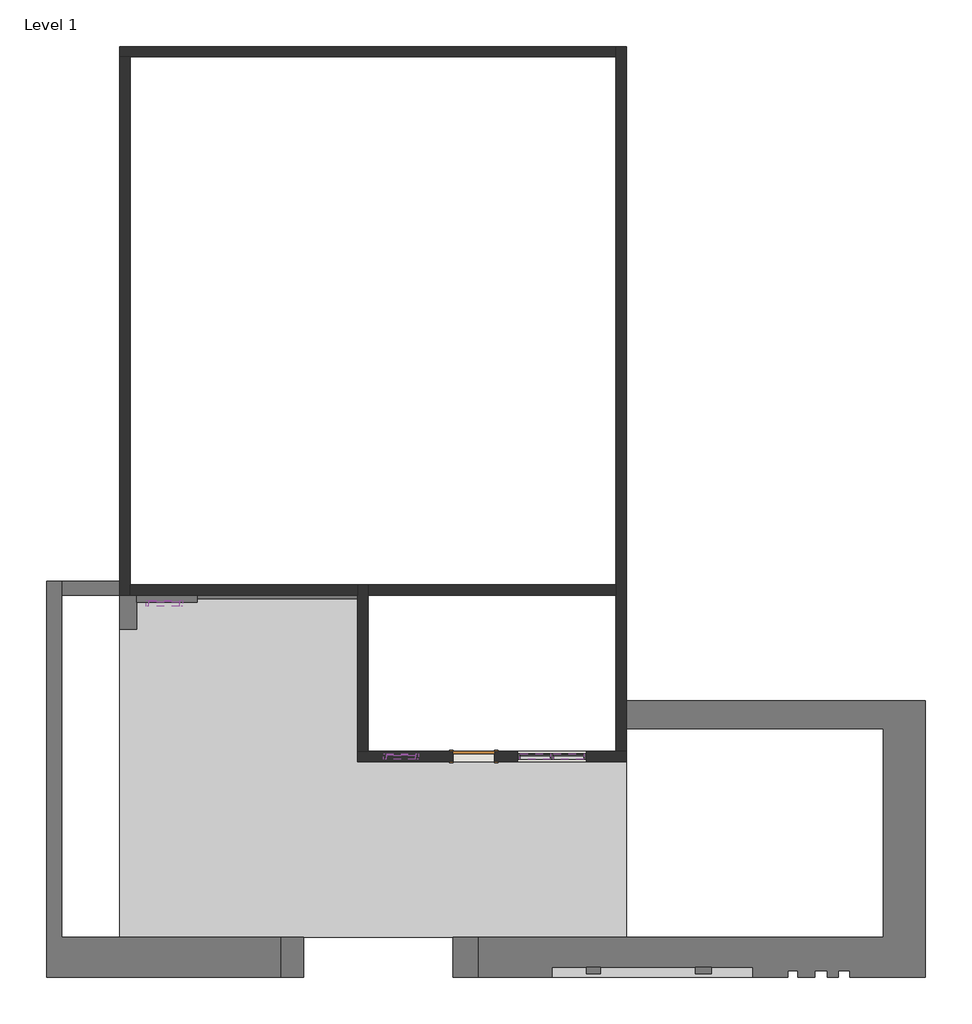
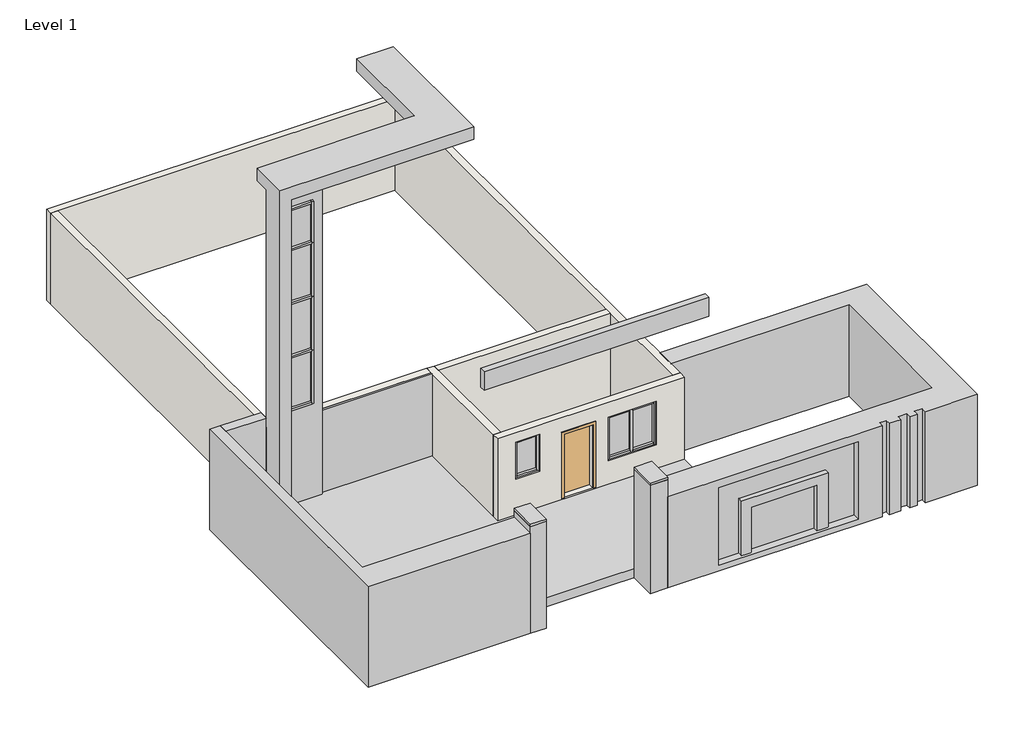
# One storey: 24 members, 7 plates, 7 walls, 4 proxies, 1 door.
"""IFC4 building model written with IfcOpenShell, lengths in millimetres."""

from ifc_helpers import new_model, si_unit, origin, origin_with_axes, place, context, project, spatial, polyline, outline, extrude, faceted_brep, transform, mapped, element, save
from components import generic_models_3_generic_models_3_20a2e421, generic_models_4_generic_models_4_e8bbcad5, generic_models_5_generic_models_5_9540ccd6, door_0ca8825f, member_c33c434a, member_9369ce3c, member_269047fe, member_5e365d0c, member_2caf7d25, member_5295ae1b, member_af550d70, member_0a83a24a, member_c6627131, system_panel_glazed_125786c9, system_panel_glazed_5a872b22, system_panel_glazed_70269732, system_panel_glazed_db295b58, system_panel_glazed_980f9714

model = new_model("IFC4")

# Units and contexts
model_context = context("Model", 3, world=origin())
ifc_project = project(units=[si_unit("LENGTHUNIT", "METRE", prefix="MILLI")], contexts=[model_context])

# Site, building, storey
site = spatial("IfcSite", under=ifc_project)
building = spatial("IfcBuilding", under=site)
storey = spatial("IfcBuildingStorey", under=building, Name="Level 1", Elevation=0.0)

# Proxies
placement = place(None, origin())
element("IfcBuildingElementProxy", 1, Name="Generic Models 1 : Generic Models 1", ObjectType="Generic Models 1 : Generic Models 1", at=placement, inside=storey, context=model_context, shape_type="Brep", body=[
    faceted_brep([(-10657.4321088, -9400.4468404, 304.8), (-15877.1321088, -9400.4468404, 304.8), (-15877.1321088, -16906.1468404, 304.8), (-4751.9321088, -16906.1468404, 304.8), (-4751.9321088, -13058.0468404, 304.8), (-10657.4321088, -13058.0468404, 304.8), (-10657.4321088, -12829.4468404, 304.8), (-10657.4321088, -13058.0468404, 0.0), (-4751.9321088, -13058.0468404, 0.0), (-4751.9321088, -16906.1468404, 0.0), (-15877.1321088, -16906.1468404, 0.0), (-15877.1321088, -9400.4468404, 0.0), (-10657.4321088, -9400.4468404, 0.0), (-10657.4321088, -12829.4468404, 0.0)], [[[0, 1, 2, 3, 4, 5, 6]], [[7, 8, 9, 10, 11, 12, 13]], [[1, 0, 12, 11]], [[2, 1, 11, 10]], [[12, 0, 6, 5, 7, 13]], [[3, 2, 10, 9]], [[4, 3, 9, 8]], [[5, 4, 8, 7]]]),
])
generic_models_3_generic_models_3_shape = generic_models_3_generic_models_3_20a2e421(model_context)
element("IfcBuildingElementProxy", 2, Name="Generic Models 3 : Generic Models 3", ObjectType="Generic Models 3 : Generic Models 3", at=placement, inside=storey, context=model_context, shape_type="MappedRepresentation", body=[
    mapped(generic_models_3_generic_models_3_shape, transform((0.0, 0.0, 0.0), x_axis=(1.0, 0.0, 0.0), y_axis=(0.0, 1.0, 0.0), z_axis=(0.0, 0.0, 1.0))),
])
generic_models_4_generic_models_4_shape = generic_models_4_generic_models_4_e8bbcad5(model_context)
element("IfcBuildingElementProxy", 3, Name="Generic Models 4 : Generic Models 4", ObjectType="Generic Models 4 : Generic Models 4", at=placement, inside=storey, context=model_context, shape_type="MappedRepresentation", body=[
    mapped(generic_models_4_generic_models_4_shape, transform((0.0, 0.0, 0.0), x_axis=(1.0, 0.0, 0.0), y_axis=(0.0, 1.0, 0.0), z_axis=(0.0, 0.0, 1.0))),
])
generic_models_5_generic_models_5_shape = generic_models_5_generic_models_5_9540ccd6(model_context)
element("IfcBuildingElementProxy", 4, Name="Generic Models 5 : Generic Models 5", ObjectType="Generic Models 5 : Generic Models 5", at=placement, inside=storey, context=model_context, shape_type="MappedRepresentation", body=[
    mapped(generic_models_5_generic_models_5_shape, transform((0.0, 0.0, 0.0), x_axis=(1.0, 0.0, 0.0), y_axis=(0.0, 1.0, 0.0), z_axis=(0.0, 0.0, 1.0))),
])

# Door
door_shape = door_0ca8825f(model_context)
element("IfcDoor", 5, ObjectType="Single-Flush : 36\" x 84\"", at=placement, inside=storey, context=model_context, shape_type="MappedRepresentation", body=[
    mapped(door_shape, transform((-8104.7321088, -12943.7468404, 355.6), x_axis=(1.0, 0.0, 0.0), y_axis=(0.0, 1.0, 0.0), z_axis=(0.0, 0.0, 1.0))),
])

# Members
member_shape = member_c33c434a(model_context)
element("IfcMember", 6, ObjectType="Rectangular Mullion : 2.5\" x 5\" rectangular", at=placement, inside=storey, context=model_context, shape_type="MappedRepresentation", body=[
    mapped(member_shape, transform((-6358.4821088, -12943.7468404, 1083.0066443), x_axis=(0.0, 0.0, -1.0), y_axis=(0.0, -1.0, 0.0), z_axis=(-1.0, 0.0, 0.0))),
])
element("IfcMember", 7, ObjectType="Rectangular Mullion : 2.5\" x 5\" rectangular", at=placement, inside=storey, context=model_context, shape_type="MappedRepresentation", body=[
    mapped(member_shape, transform((-7088.7321088, -12943.7468404, 1083.0066443), x_axis=(0.0, 0.0, -1.0), y_axis=(0.0, -1.0, 0.0), z_axis=(-1.0, 0.0, 0.0))),
])
member_2_shape = member_9369ce3c(model_context)
element("IfcMember", 8, ObjectType="Rectangular Mullion : 2.5\" x 5\" rectangular", at=placement, inside=storey, context=model_context, shape_type="MappedRepresentation", body=[
    mapped(member_2_shape, transform((-6390.2321088, -12943.7468404, 1083.0066443), x_axis=(1.0, 0.0, 0.0), y_axis=(0.0, -1.0, 0.0), z_axis=(0.0, 0.0, -1.0))),
])
element("IfcMember", 9, ObjectType="Rectangular Mullion : 2.5\" x 5\" rectangular", at=placement, inside=storey, context=model_context, shape_type="MappedRepresentation", body=[
    mapped(member_shape, transform((-6421.9821088, -12943.7468404, 2538.9721274), x_axis=(0.0, 0.0, 1.0), y_axis=(0.0, -1.0, 0.0), z_axis=(1.0, 0.0, 0.0))),
])
element("IfcMember", 10, ObjectType="Rectangular Mullion : 2.5\" x 5\" rectangular", at=placement, inside=storey, context=model_context, shape_type="MappedRepresentation", body=[
    mapped(member_shape, transform((-5691.7321088, -12943.7468404, 2538.9721274), x_axis=(0.0, 0.0, 1.0), y_axis=(0.0, -1.0, 0.0), z_axis=(1.0, 0.0, 0.0))),
])
member_3_shape = member_269047fe(model_context)
element("IfcMember", 11, ObjectType="Rectangular Mullion : 2.5\" x 5\" rectangular", at=placement, inside=storey, context=model_context, shape_type="MappedRepresentation", body=[
    mapped(member_3_shape, transform((-7152.2321088, -12943.7468404, 2538.9721274), x_axis=(-1.0, 0.0, 0.0), y_axis=(0.0, -1.0, 0.0), z_axis=(0.0, 0.0, 1.0))),
])
element("IfcMember", 12, ObjectType="Rectangular Mullion : 2.5\" x 5\" rectangular", at=placement, inside=storey, context=model_context, shape_type="MappedRepresentation", body=[
    mapped(member_3_shape, transform((-5628.2321088, -12943.7468404, 1083.0066443), x_axis=(1.0, 0.0, 0.0), y_axis=(0.0, -1.0, 0.0), z_axis=(0.0, 0.0, -1.0))),
])
member_4_shape = member_5e365d0c(model_context)
element("IfcMember", 13, ObjectType="Rectangular Mullion : 2.5\" x 5\" rectangular", at=placement, inside=storey, context=model_context, shape_type="MappedRepresentation", body=[
    mapped(member_4_shape, transform((-10022.4321088, -12943.7468404, 1497.0984453), x_axis=(0.0, 0.0, -1.0), y_axis=(0.0, -1.0, 0.0), z_axis=(-1.0, 0.0, 0.0))),
])
element("IfcMember", 14, ObjectType="Rectangular Mullion : 2.5\" x 5\" rectangular", at=placement, inside=storey, context=model_context, shape_type="MappedRepresentation", body=[
    mapped(member_4_shape, transform((-9387.4321088, -12943.7468404, 2733.8418528), x_axis=(0.0, 0.0, 1.0), y_axis=(0.0, -1.0, 0.0), z_axis=(1.0, 0.0, 0.0))),
])
member_5_shape = member_2caf7d25(model_context)
element("IfcMember", 15, ObjectType="Rectangular Mullion : 2.5\" x 5\" rectangular", at=placement, inside=storey, context=model_context, shape_type="MappedRepresentation", body=[
    mapped(member_5_shape, transform((-10085.9321088, -12943.7468404, 2733.8418528), x_axis=(-1.0, 0.0, 0.0), y_axis=(0.0, -1.0, 0.0), z_axis=(0.0, 0.0, 1.0))),
])
element("IfcMember", 16, ObjectType="Rectangular Mullion : 2.5\" x 5\" rectangular", at=placement, inside=storey, context=model_context, shape_type="MappedRepresentation", body=[
    mapped(member_5_shape, transform((-9323.9321088, -12943.7468404, 1497.0984453), x_axis=(1.0, 0.0, 0.0), y_axis=(0.0, -1.0, 0.0), z_axis=(0.0, 0.0, -1.0))),
])
member_6_shape = member_5295ae1b(model_context)
element("IfcMember", 17, ObjectType="Rectangular Mullion : 2.5\" x 5\" rectangular", at=placement, inside=storey, context=model_context, shape_type="MappedRepresentation", body=[
    mapped(member_6_shape, transform((-15305.6321088, -9579.3158046, 7104.8631502), x_axis=(-1.0, 0.0, 0.0), y_axis=(0.0, -1.0, 0.0), z_axis=(0.0, 0.0, 1.0))),
])
element("IfcMember", 18, ObjectType="Rectangular Mullion : 2.5\" x 5\" rectangular", at=placement, inside=storey, context=model_context, shape_type="MappedRepresentation", body=[
    mapped(member_6_shape, transform((-15305.6321088, -9579.3158046, 8903.6180215), x_axis=(-1.0, 0.0, 0.0), y_axis=(0.0, -1.0, 0.0), z_axis=(0.0, 0.0, 1.0))),
])
member_7_shape = member_af550d70(model_context)
element("IfcMember", 19, ObjectType="Rectangular Mullion : 2.5\" x 5\" rectangular", at=placement, inside=storey, context=model_context, shape_type="MappedRepresentation", body=[
    mapped(member_7_shape, transform((-14567.5949284, -9579.3158046, 8903.6180215), x_axis=(0.0, 0.0, 1.0), y_axis=(0.0, -1.0, 0.0), z_axis=(1.0, 0.0, 0.0))),
])
element("IfcMember", 20, ObjectType="Rectangular Mullion : 2.5\" x 5\" rectangular", at=placement, inside=storey, context=model_context, shape_type="MappedRepresentation", body=[
    mapped(member_7_shape, transform((-14567.5949284, -9579.3158046, 7104.8631502), x_axis=(0.0, 0.0, 1.0), y_axis=(0.0, -1.0, 0.0), z_axis=(1.0, 0.0, 0.0))),
])
element("IfcMember", 21, ObjectType="Rectangular Mullion : 2.5\" x 5\" rectangular", at=placement, inside=storey, context=model_context, shape_type="MappedRepresentation", body=[
    mapped(member_7_shape, transform((-14567.5949284, -9579.3158046, 5306.108279), x_axis=(0.0, 0.0, 1.0), y_axis=(0.0, -1.0, 0.0), z_axis=(1.0, 0.0, 0.0))),
])
element("IfcMember", 22, ObjectType="Rectangular Mullion : 2.5\" x 5\" rectangular", at=placement, inside=storey, context=model_context, shape_type="MappedRepresentation", body=[
    mapped(member_6_shape, transform((-14504.0949284, -9579.3158046, 5306.108279), x_axis=(1.0, 0.0, 0.0), y_axis=(0.0, -1.0, 0.0), z_axis=(0.0, 0.0, -1.0))),
])
element("IfcMember", 23, ObjectType="Rectangular Mullion : 2.5\" x 5\" rectangular", at=placement, inside=storey, context=model_context, shape_type="MappedRepresentation", body=[
    mapped(member_6_shape, transform((-14504.0949284, -9579.3158046, 7104.8631502), x_axis=(1.0, 0.0, 0.0), y_axis=(0.0, -1.0, 0.0), z_axis=(0.0, 0.0, -1.0))),
])
member_8_shape = member_0a83a24a(model_context)
element("IfcMember", 24, ObjectType="Rectangular Mullion : 2.5\" x 5\" rectangular", at=placement, inside=storey, context=model_context, shape_type="MappedRepresentation", body=[
    mapped(member_8_shape, transform((-14567.5949284, -9579.3158046, 10275.2180215), x_axis=(0.0, 0.0, 1.0), y_axis=(0.0, -1.0, 0.0), z_axis=(1.0, 0.0, 0.0))),
])
member_9_shape = member_c6627131(model_context)
element("IfcMember", 25, ObjectType="Rectangular Mullion : 2.5\" x 5\" rectangular", at=placement, inside=storey, context=model_context, shape_type="MappedRepresentation", body=[
    mapped(member_9_shape, transform((-15305.6321088, -9579.3158046, 10275.2180215), x_axis=(-1.0, 0.0, 0.0), y_axis=(0.0, -1.0, 0.0), z_axis=(0.0, 0.0, 1.0))),
])
element("IfcMember", 26, ObjectType="Rectangular Mullion : 2.5\" x 5\" rectangular", at=placement, inside=storey, context=model_context, shape_type="MappedRepresentation", body=[
    mapped(member_9_shape, transform((-14504.0949284, -9579.3158046, 8903.6180215), x_axis=(1.0, 0.0, 0.0), y_axis=(0.0, -1.0, 0.0), z_axis=(0.0, 0.0, -1.0))),
])
element("IfcMember", 27, ObjectType="Rectangular Mullion : 2.5\" x 5\" rectangular", at=placement, inside=storey, context=model_context, shape_type="MappedRepresentation", body=[
    mapped(member_8_shape, transform((-15242.1321088, -9579.3158046, 3507.3534077), x_axis=(0.0, 0.0, -1.0), y_axis=(0.0, -1.0, 0.0), z_axis=(-1.0, 0.0, 0.0))),
])
element("IfcMember", 28, ObjectType="Rectangular Mullion : 2.5\" x 5\" rectangular", at=placement, inside=storey, context=model_context, shape_type="MappedRepresentation", body=[
    mapped(member_6_shape, transform((-15305.6321088, -9579.3158046, 5306.108279), x_axis=(-1.0, 0.0, 0.0), y_axis=(0.0, -1.0, 0.0), z_axis=(0.0, 0.0, 1.0))),
])
element("IfcMember", 29, ObjectType="Rectangular Mullion : 2.5\" x 5\" rectangular", at=placement, inside=storey, context=model_context, shape_type="MappedRepresentation", body=[
    mapped(member_6_shape, transform((-14504.0949284, -9579.3158046, 3507.3534077), x_axis=(1.0, 0.0, 0.0), y_axis=(0.0, -1.0, 0.0), z_axis=(0.0, 0.0, -1.0))),
])

# Plates
system_panel_glazed_shape = system_panel_glazed_125786c9(model_context)
element("IfcPlate", 30, ObjectType="System Panel : Glazed", at=placement, inside=storey, context=model_context, shape_type="MappedRepresentation", body=[
    mapped(system_panel_glazed_shape, transform((-6755.3571088, -12943.7468404, 1146.5066443), x_axis=(1.0, 0.0, 0.0), y_axis=(0.0, 1.0, 0.0), z_axis=(0.0, 0.0, 1.0))),
])
element("IfcPlate", 31, ObjectType="System Panel : Glazed", at=placement, inside=storey, context=model_context, shape_type="MappedRepresentation", body=[
    mapped(system_panel_glazed_shape, transform((-6025.1071088, -12943.7468404, 1146.5066443), x_axis=(1.0, 0.0, 0.0), y_axis=(0.0, 1.0, 0.0), z_axis=(0.0, 0.0, 1.0))),
])
system_panel_glazed_2_shape = system_panel_glazed_5a872b22(model_context)
element("IfcPlate", 32, ObjectType="System Panel : Glazed", at=placement, inside=storey, context=model_context, shape_type="MappedRepresentation", body=[
    mapped(system_panel_glazed_2_shape, transform((-9704.9321088, -12943.7468404, 1560.5984453), x_axis=(1.0, 0.0, 0.0), y_axis=(0.0, 1.0, 0.0), z_axis=(0.0, 0.0, 1.0))),
])
system_panel_glazed_3_shape = system_panel_glazed_70269732(model_context)
element("IfcPlate", 33, ObjectType="System Panel : Glazed", at=placement, inside=storey, context=model_context, shape_type="MappedRepresentation", body=[
    mapped(system_panel_glazed_3_shape, transform((-14904.8635186, -9579.3158046, 7136.6131502), x_axis=(1.0, 0.0, 0.0), y_axis=(0.0, 1.0, 0.0), z_axis=(0.0, 0.0, 1.0))),
])
element("IfcPlate", 34, ObjectType="System Panel : Glazed", at=placement, inside=storey, context=model_context, shape_type="MappedRepresentation", body=[
    mapped(system_panel_glazed_3_shape, transform((-14904.8635186, -9579.3158046, 5337.858279), x_axis=(1.0, 0.0, 0.0), y_axis=(0.0, 1.0, 0.0), z_axis=(0.0, 0.0, 1.0))),
])
system_panel_glazed_4_shape = system_panel_glazed_db295b58(model_context)
element("IfcPlate", 35, ObjectType="System Panel : Glazed", at=placement, inside=storey, context=model_context, shape_type="MappedRepresentation", body=[
    mapped(system_panel_glazed_4_shape, transform((-14904.8635186, -9579.3158046, 8935.3680215), x_axis=(1.0, 0.0, 0.0), y_axis=(0.0, 1.0, 0.0), z_axis=(0.0, 0.0, 1.0))),
])
system_panel_glazed_5_shape = system_panel_glazed_980f9714(model_context)
element("IfcPlate", 36, ObjectType="System Panel : Glazed", at=placement, inside=storey, context=model_context, shape_type="MappedRepresentation", body=[
    mapped(system_panel_glazed_5_shape, transform((-14904.8635186, -9579.3158046, 3570.8534077), x_axis=(1.0, 0.0, 0.0), y_axis=(0.0, 1.0, 0.0), z_axis=(0.0, 0.0, 1.0))),
])

# Walls
element("IfcWall", 37, ObjectType="9\"", at=placement, inside=storey, context=model_context, shape_type="Brep", body=[
    faceted_brep([(-4751.9321088, -12829.4468404, 0.0), (-4751.9321088, 2639.1531596, 0.0), (-4751.9321088, 2639.1531596, 3048.0), (-4751.9321088, -12829.4468404, 3048.0), (-4980.5321088, -12829.4468404, 0.0), (-4980.5321088, -12829.4468404, 3048.0), (-4980.5321088, -9400.4468404, 3048.0), (-4980.5321088, -9171.8468404, 3048.0), (-4980.5321088, 2410.5531596, 3048.0), (-4980.5321088, 2639.1531596, 3048.0), (-4980.5321088, 2639.1531596, 0.0), (-4980.5321088, 2410.5531596, 0.0), (-4980.5321088, -9171.8468404, 0.0), (-4980.5321088, -9400.4468404, 0.0)], [[[0, 1, 2, 3]], [[4, 5, 6, 7, 8, 9, 10, 11, 12, 13]], [[1, 0, 4, 13, 12, 11, 10]], [[3, 2, 9, 8, 7, 6, 5]], [[0, 3, 5, 4]], [[2, 1, 10, 9]]]),
])
element("IfcWall", 38, ObjectType="9\"", at=placement, inside=storey, context=model_context, shape_type="Brep", body=[
    faceted_brep([(-4980.5321088, 2639.1531596, 0.0), (-15877.1321088, 2639.1531596, 0.0), (-15877.1321088, 2639.1531596, 3048.0), (-4980.5321088, 2639.1531596, 3048.0), (-4980.5321088, 2410.5531596, 0.0), (-4980.5321088, 2410.5531596, 3048.0), (-15648.5321088, 2410.5531596, 3048.0), (-15877.1321088, 2410.5531596, 3048.0), (-15877.1321088, 2410.5531596, 0.0), (-15648.5321088, 2410.5531596, 0.0)], [[[0, 1, 2, 3]], [[4, 5, 6, 7, 8, 9]], [[1, 0, 4, 9, 8]], [[3, 2, 7, 6, 5]], [[0, 3, 5, 4]], [[2, 1, 8, 7]]]),
])
element("IfcWall", 39, ObjectType="9\"", at=placement, inside=storey, context=model_context, shape_type="Brep", body=[
    faceted_brep([(-15877.1321088, 2410.5531596, 0.0), (-15877.1321088, -9400.4468404, 0.0), (-15877.1321088, -9400.4468404, 3048.0), (-15877.1321088, 2410.5531596, 3048.0), (-15648.5321088, 2410.5531596, 0.0), (-15648.5321088, 2410.5531596, 3048.0), (-15648.5321088, -9171.8468404, 3048.0), (-15648.5321088, -9400.4468404, 3048.0), (-15648.5321088, -9400.4468404, 0.0), (-15648.5321088, -9171.8468404, 0.0)], [[[0, 1, 2, 3]], [[4, 5, 6, 7, 8, 9]], [[1, 0, 4, 9, 8]], [[2, 1, 8, 7]], [[3, 2, 7, 6, 5]], [[0, 3, 5, 4]]]),
])
element("IfcWall", 40, ObjectType="9\"", at=placement, inside=storey, context=model_context, shape_type="Brep", body=[
    faceted_brep([(-10428.8321088, -12829.4468404, 0.0), (-10428.8321088, -9400.4468404, 0.0), (-10428.8321088, -9171.8468404, 0.0), (-10428.8321088, -9171.8468404, 3048.0), (-10428.8321088, -9400.4468404, 3048.0), (-10428.8321088, -12829.4468404, 3048.0), (-10657.4321088, -12829.4468404, 0.0), (-10657.4321088, -12829.4468404, 3048.0), (-10657.4321088, -9400.4468404, 3048.0), (-10657.4321088, -9171.8468404, 3048.0), (-10657.4321088, -9171.8468404, 0.0), (-10657.4321088, -9400.4468404, 0.0)], [[[0, 1, 2, 3, 4, 5]], [[6, 7, 8, 9, 10, 11]], [[2, 1, 0, 6, 11, 10]], [[5, 4, 3, 9, 8, 7]], [[0, 5, 7, 6]], [[3, 2, 10, 9]]]),
])
element("IfcWall", 41, ObjectType="9\"", at=placement, inside=storey, context=model_context, shape_type="SweptSolid", body=[
    extrude(outline(polyline([(-4980.5321088, -9400.4468404), (-10428.8321088, -9400.4468404), (-10428.8321088, -9171.8468404), (-4980.5321088, -9171.8468404), (-4980.5321088, -9400.4468404)])), origin_with_axes(), (0.0, 0.0, 1.0), 3048.0),
])
element("IfcWall", 42, ObjectType="9\"", at=placement, inside=storey, context=model_context, shape_type="SweptSolid", body=[
    extrude(outline(polyline([(-15648.5321088, -9171.8468404), (-10657.4321088, -9171.8468404), (-10657.4321088, -9400.4468404), (-15648.5321088, -9400.4468404), (-15648.5321088, -9171.8468404)])), origin_with_axes(), (0.0, 0.0, 1.0), 3048.0),
])
element("IfcWall", 43, ObjectType="9\"", at=placement, inside=storey, context=model_context, shape_type="Brep", body=[
    faceted_brep([(-10657.4321088, -13058.0468404, 0.0), (-4751.9321088, -13058.0468404, 0.0), (-4751.9321088, -13058.0468404, 3048.0), (-10657.4321088, -13058.0468404, 3048.0), (-10085.9321088, -13058.0468404, 1497.0984453), (-10085.9321088, -13058.0468404, 2733.8418528), (-9323.9321088, -13058.0468404, 2733.8418528), (-9323.9321088, -13058.0468404, 1497.0984453), (-7647.5321088, -13058.0468404, 355.6), (-8561.9321088, -13058.0468404, 355.6), (-8561.9321088, -13058.0468404, 2489.2), (-7647.5321088, -13058.0468404, 2489.2), (-7152.2321088, -13058.0468404, 1083.0066443), (-7152.2321088, -13058.0468404, 2538.9721274), (-5628.2321088, -13058.0468404, 2538.9721274), (-5628.2321088, -13058.0468404, 1083.0066443), (-4751.9321088, -12829.4468404, 0.0), (-4980.5321088, -12829.4468404, 0.0), (-10428.8321088, -12829.4468404, 0.0), (-10657.4321088, -12829.4468404, 0.0), (-10657.4321088, -12829.4468404, 3048.0), (-10428.8321088, -12829.4468404, 3048.0), (-4980.5321088, -12829.4468404, 3048.0), (-4751.9321088, -12829.4468404, 3048.0), (-10085.9321088, -12829.4468404, 2733.8418528), (-10085.9321088, -12829.4468404, 1497.0984453), (-9323.9321088, -12829.4468404, 1497.0984453), (-9323.9321088, -12829.4468404, 2733.8418528), (-8561.9321088, -12829.4468404, 355.6), (-7647.5321088, -12829.4468404, 355.6), (-7647.5321088, -12829.4468404, 2489.2), (-8561.9321088, -12829.4468404, 2489.2), (-7152.2321088, -12829.4468404, 2538.9721274), (-7152.2321088, -12829.4468404, 1083.0066443), (-5628.2321088, -12829.4468404, 1083.0066443), (-5628.2321088, -12829.4468404, 2538.9721274)], [[[0, 1, 2, 3], [4, 5, 6, 7], [8, 9, 10, 11], [12, 13, 14, 15]], [[16, 17, 18, 19, 20, 21, 22, 23], [24, 25, 26, 27], [28, 29, 30, 31], [32, 33, 34, 35]], [[1, 0, 19, 18, 17, 16]], [[3, 2, 23, 22, 21, 20]], [[0, 3, 20, 19]], [[2, 1, 16, 23]], [[24, 5, 4, 25]], [[5, 24, 27, 6]], [[6, 27, 26, 7]], [[25, 4, 7, 26]], [[29, 28, 9, 8]], [[30, 29, 8, 11]], [[31, 30, 11, 10]], [[28, 31, 10, 9]], [[12, 33, 32, 13]], [[13, 32, 35, 14]], [[14, 35, 34, 15]], [[33, 12, 15, 34]]]),
])

save(model, "model.ifc")

# Revit data of these elements
# Type "Single-Flush : 36\" x 84\""
#   Type Mark = "1"
#   Construction Type Id = "MDOOR"
#   Assembly Code = "C1020"
#   Analytic Construction = "Metal"
#   Thickness = 0' - 2"
#   Heat Transfer Coefficient (U) = 0.651978 BTU/(h·ft²·°F)
#   Height = 7' - 0"
#   Trim Projection Ext = 0' - 1"
#   Trim Projection Int = 0' - 1"
#   Trim Width = 0' - 3"
#   Width = 3' - 0"
#   Define Thermal Properties by = 1
#   Define Thermal Properties by = 1
#   Door Material = Door - Panel
#   Frame Material = Door - Frame
#   Visual Light Transmittance = 0
#   Solar Heat Gain Coefficient = 0
#   Function = (empty or 0)
#   Wall Closure = (empty or 0)
# Type "Rectangular Mullion : 2.5\" x 5\" rectangular"
#   built-in parameter 1007304 = 0.416667 (stored number, unit not read)
#   built-in parameter 1007301 = 0.104167 (stored number, unit not read)
#   built-in parameter 1007300 = 0.104167 (stored number, unit not read)
# Type "System Panel : Glazed"
#   Construction Type Id = "GSP4R"
#   Analytic Construction = "1/8 in Pilkington single glazing"
#   Visual Light Transmittance = 0.9
#   Solar Heat Gain Coefficient = 0.86
#   Heat Transfer Coefficient (U) = 1.18115 BTU/(h·ft²·°F)
#   Define Thermal Properties by = 1
# Type "9\""
#   Assembly Code = "B2010"
#   Layers, outside or top first: 0' - 9" no material (function 1)
# Element 1 (IfcBuildingElementProxy, "Generic Models 1 : Generic Models 1")
#   Phase Created = New Construction
# Element 2 (IfcBuildingElementProxy, "Generic Models 3 : Generic Models 3")
#   Phase Created = New Construction
# Element 3 (IfcBuildingElementProxy, "Generic Models 4 : Generic Models 4")
#   Phase Created = New Construction
# Element 4 (IfcBuildingElementProxy, "Generic Models 5 : Generic Models 5")
#   Phase Created = New Construction
# Element 5 (IfcDoor, "Single-Flush : 36\" x 84\"")
#   Phase Created = New Construction
#   Materials on its faces: "Door - Frame", "Door - Panel"
# Elements 6, 7, 8, 9, 10, 11, 12, 13, 14, 15, 16, 17, 18, 19, 20, 21, 22, 23, 24, 25, 26, 27, 28, 29 (IfcMember, "Rectangular Mullion : 2.5\" x 5\" rectangular")
#   Phase Created = New Construction
#   Materials on its faces: "Aluminum"
# Elements 30, 31, 32, 33, 34, 35, 36 (IfcPlate, "System Panel : Glazed")
#   Phase Created = New Construction
#   Materials on its faces: "Glass"
# Elements 37, 38, 39, 40, 41, 42, 43 (IfcWall, "9\"")
#   Top Offset = 0' - 0"
#   Base Offset = 0' - 0"
#   Unconnected Height = 10' - 0"
#   wall height = 10' - 0"
#   Phase Created = New Construction
#   Base Constraint = Level 1
#   Materials on its faces: "Default Wall"
# Materials
#   "Door - Panel": class "Wood", colour RGB 210 159 95, transparency 0, Cost = 0
#   "Door - Frame": colour RGB 118 70 51, transparency 0, Cost = 0
#   "Aluminum": class "Metal", colour RGB 247 247 247, transparency 0, Description = "Aluminum 6061", Cost = 0
#   "Glass": class "Glass", colour RGB 0 128 192, transparency 0.75, Description = "Soda Lime Glass", Cost = 0
#   "Default Wall": colour RGB 128 128 128, transparency 0, Cost = 0
